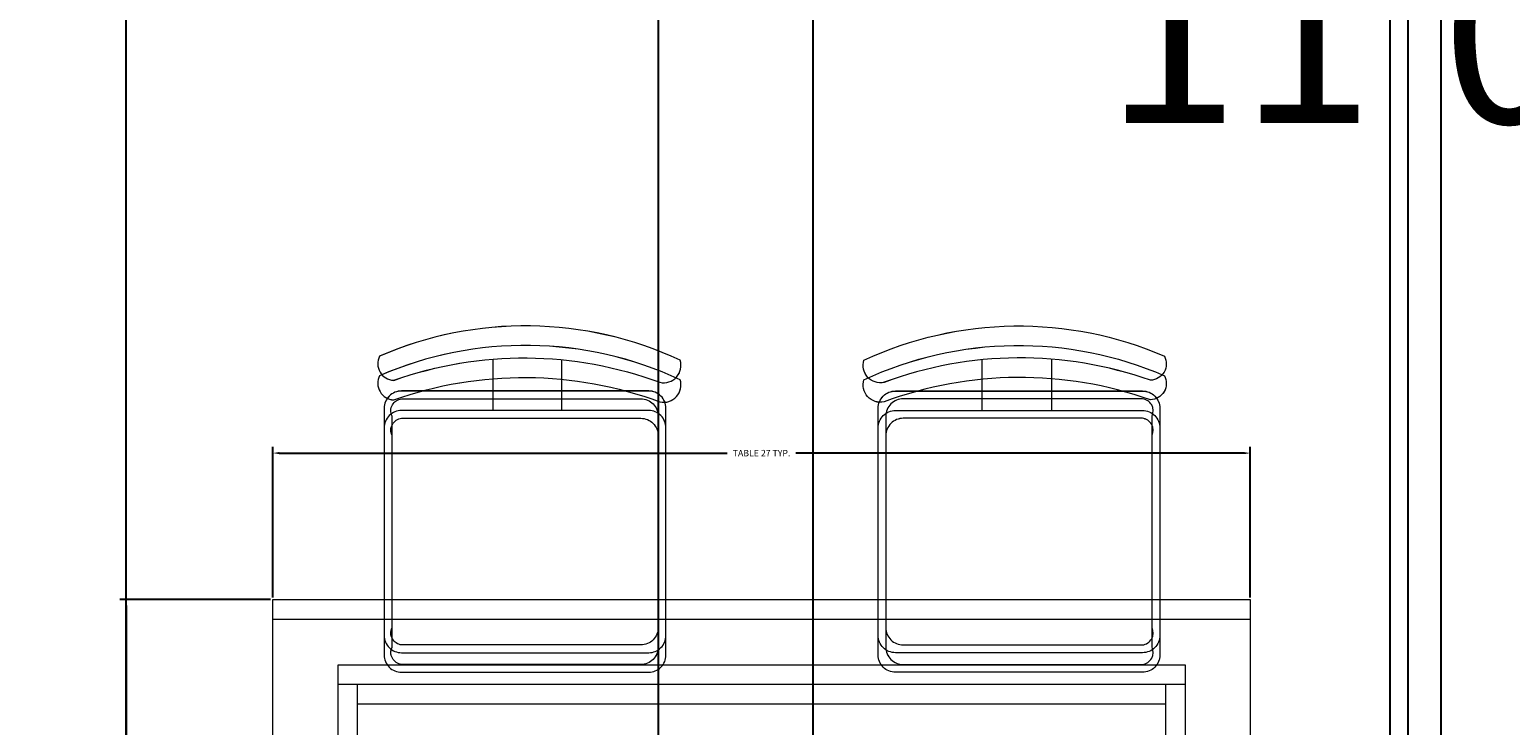
# Model space of a CAD drawing. Units: inches. Extents: x 2063 to 2617, y 1299 to 2210.
# Tile 11 of 22: x 2242 to 2284, y 1925 to 1945. Entities that reach past the tile are written whole.
import ezdxf

# ---------------------------------------------------------------- set-up
doc = ezdxf.new("R2010")
doc.units = ezdxf.units.IN
for name, color, linetype, lineweight in [('A-ANNO-DIMS', 2, 'Continuous', 18), ('A-AREA-IDEN', 7, 'Continuous', 18), ('A-FURN', 8, 'Continuous', 18)]:
    doc.layers.add(name, color=color, linetype=linetype, lineweight=lineweight)
doc.layers.add('A-WALL-PATT', color=215, linetype='Continuous', lineweight=13, true_color=0xa953a0)
doc.styles.get("Standard").update_dxf_attribs({"font": 'arial.ttf'})
doc.dimstyles.get("Standard").update_dxf_attribs({"dimtxt": 0.18, "dimasz": 0.18, "dimexe": 0.18, "dimexo": 0.0625, "dimgap": 0.09, "dimtad": 0, "dimtih": 1, "dimtoh": 1, "dimdec": 4, "dimzin": 0, "dimdsep": 46, "dimtxsty": 'Standard', "dimcen": 0.09, "dimadec": 0, "dimazin": 0, "dimtfac": 1, "dimtdec": 4, "dimtofl": 0, "dimtmove": 0, "dimatfit": 3, "dimfxl": 1, "dimtolj": 1, "dimtzin": 0, "dimarcsym": 0})

# ---------------------------------------------------------------- blocks, each defined once
blk = doc.blocks.new('TABLE-DINING')
for points in [[(0, 17.017), (27.446, 17.017), (27.446, 0.549), (0, 0.549)], [(0, 17.017), (27.446, 17.017), (27.446, 0.549), (0, 0.549)], [(0, 17.016), (27.446, 17.016), (27.446, 0.549), (0, 0.549)], [(0, 17.016), (27.446, 17.016), (27.446, 0.549), (0, 0.549)], [(0, 16.468), (27.446, 16.468), (27.446, 0), (0, 0)], [(0, 16.468), (27.446, 16.468), (27.446, 0), (0, 0)], [(0, 16.467), (27.446, 16.467), (27.446, 0), (0, 0)], [(0, 16.467), (27.446, 16.467), (27.446, 0), (0, 0)], [(1.83, 15.187), (25.616, 15.187), (25.616, 2.379), (1.83, 2.379)], [(1.83, 15.187), (25.616, 15.187), (25.616, 2.379), (1.83, 2.379)], [(1.83, 15.187), (25.616, 15.187), (25.616, 2.379), (1.83, 2.379)], [(1.83, 15.187), (25.616, 15.187), (25.616, 2.379), (1.83, 2.379)], [(1.83, 14.638), (25.616, 14.638), (25.616, 1.83), (1.83, 1.83)], [(1.83, 14.638), (25.616, 14.638), (25.616, 1.83), (1.83, 1.83)], [(1.83, 14.638), (25.616, 14.638), (25.616, 1.83), (1.83, 1.83)], [(1.83, 14.638), (25.616, 14.638), (25.616, 1.83), (1.83, 1.83)], [(2.379, 14.638), (25.067, 14.638), (25.067, 2.928), (2.379, 2.928)], [(2.379, 14.638), (25.067, 14.638), (25.067, 2.927), (2.379, 2.927)], [(2.379, 14.638), (25.067, 14.638), (25.067, 2.928), (2.379, 2.928)], [(2.379, 14.638), (25.067, 14.638), (25.067, 2.927), (2.379, 2.927)], [(2.379, 14.089), (25.067, 14.089), (25.067, 2.379), (2.379, 2.379)], [(2.379, 14.089), (25.067, 14.089), (25.067, 2.379), (2.379, 2.379)], [(2.379, 14.089), (25.067, 14.089), (25.067, 2.379), (2.379, 2.379)], [(2.379, 14.089), (25.067, 14.089), (25.067, 2.379), (2.379, 2.379)]]:
    blk.add_lwpolyline(points, close=True)
blk = doc.blocks.new('CHAIR-DINING')
for points in [[(0.449, 8.202, -0.175809), (7.924, 8.145, 0.578392), (8.491, 8.768, 0.214524), (0.052, 8.881, 0.552014), (0.449, 8.202, -0.065079)], [(0.449, 8.201, -0.175809), (7.924, 8.145, 0.578392), (8.491, 8.767, 0.214524), (0.053, 8.881, 0.552014), (0.449, 8.201, -0.065079)], [(0.449, 8.202, -0.175809), (7.924, 8.145, 0.578392), (8.491, 8.768, 0.214524), (0.052, 8.881, 0.552014), (0.449, 8.202, -0.065079)], [(0.449, 8.201, -0.175809), (7.924, 8.145, 0.578392), (8.491, 8.767, 0.214524), (0.053, 8.881, 0.552014), (0.449, 8.201, -0.065079)], [(0.449, 7.653, -0.175809), (7.924, 7.596, 0.578392), (8.491, 8.219, 0.214524), (0.052, 8.332, 0.552014), (0.449, 7.653, -0.065079)], [(0.449, 7.652, -0.175809), (7.924, 7.596, 0.578392), (8.491, 8.218, 0.214524), (0.053, 8.332, 0.552014), (0.449, 7.652, -0.065079)], [(0.449, 7.653, -0.175809), (7.924, 7.596, 0.578392), (8.491, 8.219, 0.214524), (0.052, 8.332, 0.552014), (0.449, 7.653, -0.065079)], [(0.449, 7.652, -0.175809), (7.924, 7.596, 0.578392), (8.491, 8.218, 0.214524), (0.053, 8.332, 0.552014), (0.449, 7.652, -0.065079)], [(5.17, 7.902), (5.17, 8.779, -0.064759)], [(5.17, 7.901), (5.17, 8.779, -0.064759)], [(5.17, 7.902), (5.17, 8.779, -0.064759)], [(5.17, 7.901), (5.17, 8.779, -0.064759)], [(7.607, 7.902), (0.667, 7.902, 0.414214), (0.182, 7.416), (0.182, 1.035, 0.414214), (0.667, 0.549), (7.607, 0.549, 0.414214), (8.093, 1.035), (8.093, 7.416, 0.414214), (7.607, 7.902)], [(7.607, 7.902), (0.667, 7.902, 0.414214), (0.182, 7.416), (0.182, 1.035, 0.414214), (0.667, 0.549), (7.607, 0.549, 0.414214), (8.093, 1.035), (8.093, 7.416, 0.414214), (7.607, 7.902)], [(7.607, 7.901), (0.667, 7.901, 0.414214), (0.182, 7.416), (0.182, 1.035, 0.414214), (0.667, 0.549), (7.607, 0.549, 0.414214), (8.093, 1.035), (8.093, 7.416, 0.414214), (7.607, 7.901)], [(7.607, 7.901), (0.667, 7.901, 0.414214), (0.182, 7.416), (0.182, 1.035, 0.414214), (0.667, 0.549), (7.607, 0.549, 0.414214), (8.093, 1.035), (8.093, 7.416, 0.414214), (7.607, 7.901)], [(5.17, 7.353), (5.17, 8.23, -0.064759)], [(5.17, 7.352), (5.17, 8.23, -0.064759)], [(5.17, 7.353), (5.17, 8.23, -0.064759)], [(5.17, 7.352), (5.17, 8.23, -0.064759)], [(7.607, 7.353), (0.667, 7.353, 0.414214), (0.182, 6.867), (0.182, 0.486, 0.414214), (0.667, 0), (7.607, 0, 0.414214), (8.093, 0.486), (8.093, 6.867, 0.414214), (7.607, 7.353)], [(7.607, 7.353), (0.667, 7.353, 0.414214), (0.182, 6.867), (0.182, 0.486, 0.414214), (0.667, 0), (7.607, 0, 0.414214), (8.093, 0.486), (8.093, 6.867, 0.414214), (7.607, 7.353)], [(7.607, 7.352), (0.667, 7.352, 0.414214), (0.182, 6.867), (0.182, 0.486, 0.414214), (0.667, 0), (7.607, 0, 0.414214), (8.093, 0.486), (8.093, 6.867, 0.414214), (7.607, 7.352)], [(7.607, 7.352), (0.667, 7.352, 0.414214), (0.182, 6.867), (0.182, 0.486, 0.414214), (0.667, 0), (7.607, 0, 0.414214), (8.093, 0.486), (8.093, 6.867, 0.414214), (7.607, 7.352)]]:
    blk.add_lwpolyline(points, format="xyb")
for points in [[(3.227, 8.795), (3.227, 7.902)], [(3.227, 8.795), (3.227, 7.901)], [(3.227, 8.795), (3.227, 7.902)], [(3.227, 8.795), (3.227, 7.901)], [(3.227, 8.246), (3.227, 7.353)], [(3.227, 8.246), (3.227, 7.352)], [(3.227, 8.246), (3.227, 7.353)], [(3.227, 8.246), (3.227, 7.352)]]:
    blk.add_lwpolyline(points)
for points in [[(0.67, 7.683), (7.388, 7.683, -0.414214), (7.874, 7.197), (7.874, 1.254, -0.414214), (7.388, 0.768), (0.67, 0.768, -0.512069), (0.4, 1.254), (0.4, 7.197, -0.512069)], [(0.67, 7.683), (7.388, 7.683, -0.414214), (7.874, 7.197), (7.874, 1.253, -0.414214), (7.388, 0.768), (0.67, 0.768, -0.512069), (0.4, 1.253), (0.4, 7.197, -0.512069)], [(0.67, 7.683), (7.388, 7.683, -0.414214), (7.874, 7.197), (7.874, 1.254, -0.414214), (7.388, 0.768), (0.67, 0.768, -0.512069), (0.4, 1.254), (0.4, 7.197, -0.512069)], [(0.67, 7.683), (7.388, 7.683, -0.414214), (7.874, 7.197), (7.874, 1.253, -0.414214), (7.388, 0.768), (0.67, 0.768, -0.512069), (0.4, 1.253), (0.4, 7.197, -0.512069)], [(0.67, 7.134), (7.388, 7.134, -0.414214), (7.874, 6.648), (7.874, 0.705, -0.414214), (7.388, 0.219), (0.67, 0.219, -0.512069), (0.4, 0.705), (0.4, 6.648, -0.512069)], [(0.67, 7.134), (7.388, 7.134, -0.414214), (7.874, 6.648), (7.874, 0.704, -0.414214), (7.388, 0.219), (0.67, 0.219, -0.512069), (0.4, 0.704), (0.4, 6.648, -0.512069)], [(0.67, 7.134), (7.388, 7.134, -0.414214), (7.874, 6.648), (7.874, 0.705, -0.414214), (7.388, 0.219), (0.67, 0.219, -0.512069), (0.4, 0.705), (0.4, 6.648, -0.512069)], [(0.67, 7.134), (7.388, 7.134, -0.414214), (7.874, 6.648), (7.874, 0.704, -0.414214), (7.388, 0.219), (0.67, 0.219, -0.512069), (0.4, 0.704), (0.4, 6.648, -0.512069)]]:
    blk.add_lwpolyline(points, format="xyb", close=True)
blk = doc.blocks.new('*D25')
at = {"layer": 'A-ANNO-DIMS', "color": 0, "lineweight": -2, "transparency": 16777216}
for p, q in [((2248.983, 1928.797), (2248.983, 1933.031)), ((2276.429, 1928.797), (2276.429, 1933.031)), ((2249.163, 1932.851), (2261.742, 1932.851)), ((2276.249, 1932.851), (2263.67, 1932.851))]:
    blk.add_line(p, q, dxfattribs=at)
at = {"layer": 'A-ANNO-DIMS', "color": 0, "transparency": 16777216}
for points in [[(2249.163, 1932.881), (2249.163, 1932.821), (2248.983, 1932.851)], [(2276.249, 1932.881), (2276.249, 1932.821), (2276.429, 1932.851)]]:
    blk.add_solid(points, dxfattribs=at)
at = {"layer": 'Defpoints', "color": 0, "transparency": 16777216}
for p in [(2276.429, 1932.851), (2248.983, 1928.735), (2276.429, 1928.735)]:
    blk.add_point(p, dxfattribs=at)
at = {"layer": 'A-ANNO-DIMS', "color": 0, "transparency": 16777216, "insert": (2262.706, 1932.851), "char_height": 0.18, "attachment_point": 5}
blk.add_mtext('\\A1;TABLE 27 TYP.', dxfattribs=at)
blk = doc.blocks.new('*D26')
at = {"layer": 'A-ANNO-DIMS', "color": 0, "lineweight": -2, "transparency": 16777216}
for p, q in [((2248.921, 1928.735), (2244.686, 1928.735)), ((2244.866, 1928.555), (2244.866, 1920.407)), ((2244.866, 1911.898), (2244.866, 1920.046)), ((2248.921, 1911.718), (2244.686, 1911.718))]:
    blk.add_line(p, q, dxfattribs=at)
at = {"layer": 'A-ANNO-DIMS', "color": 0, "transparency": 16777216}
for points in [[(2244.836, 1928.555), (2244.896, 1928.555), (2244.866, 1928.735)], [(2244.836, 1911.898), (2244.896, 1911.898), (2244.866, 1911.718)]]:
    blk.add_solid(points, dxfattribs=at)
at = {"layer": 'Defpoints', "color": 0, "transparency": 16777216}
for p in [(2244.866, 1928.735), (2248.983, 1928.735), (2248.983, 1911.718)]:
    blk.add_point(p, dxfattribs=at)
at = {"layer": 'A-ANNO-DIMS', "color": 0, "transparency": 16777216, "insert": (2244.866, 1920.226), "char_height": 0.18, "attachment_point": 5}
blk.add_mtext('\\A1;17 TYP.', dxfattribs=at)
blk = doc.blocks.new('*D50')
at = {"layer": 'A-ANNO-DIMS', "color": 0, "lineweight": -2, "transparency": 16777216}
for p, q in [((2264.144, 2124.25), (2264.144, 1317.702)), ((2280.348, 2124.25), (2280.348, 1317.702)), ((2264.324, 1317.882), (2271.791, 1317.882)), ((2280.168, 1317.882), (2272.701, 1317.882))]:
    blk.add_line(p, q, dxfattribs=at)
at = {"layer": 'A-ANNO-DIMS', "color": 0, "transparency": 16777216}
for points in [[(2264.324, 1317.912), (2264.324, 1317.852), (2264.144, 1317.882)], [(2280.168, 1317.912), (2280.168, 1317.852), (2280.348, 1317.882)]]:
    blk.add_solid(points, dxfattribs=at)
at = {"layer": 'Defpoints', "color": 0, "transparency": 16777216}
for p in [(2264.144, 2124.312), (2280.348, 2124.312), (2280.348, 1317.882)]:
    blk.add_point(p, dxfattribs=at)
at = {"layer": 'A-ANNO-DIMS', "color": 0, "transparency": 16777216, "insert": (2272.246, 1317.882), "char_height": 0.18, "attachment_point": 5}
blk.add_mtext('\\A1;16.204', dxfattribs=at)
blk = doc.blocks.new('*D62')
at = {"layer": 'A-ANNO-DIMS', "color": 0, "lineweight": -2, "transparency": 16777216}
for p, q in [((2259.809, 1437.875), (2259.809, 2170.742)), ((2259.989, 2170.562), (2270.403, 2170.562)), ((2281.608, 2170.562), (2271.194, 2170.562)), ((2281.788, 1437.875), (2281.788, 2170.742))]:
    blk.add_line(p, q, dxfattribs=at)
at = {"layer": 'A-ANNO-DIMS', "color": 0, "transparency": 16777216}
for points in [[(2259.989, 2170.592), (2259.989, 2170.532), (2259.809, 2170.562)], [(2281.608, 2170.592), (2281.608, 2170.532), (2281.788, 2170.562)]]:
    blk.add_solid(points, dxfattribs=at)
at = {"layer": 'Defpoints', "color": 0, "transparency": 16777216}
for p in [(2281.788, 2170.562), (2259.809, 1437.812), (2281.788, 1437.812)]:
    blk.add_point(p, dxfattribs=at)
at = {"layer": 'A-ANNO-DIMS', "color": 0, "transparency": 16777216, "insert": (2270.798, 2170.562), "char_height": 0.18, "attachment_point": 5}
blk.add_mtext('\\A1;21.98', dxfattribs=at)
blk = doc.blocks.new('*D63')
at = {"layer": 'A-ANNO-DIMS', "color": 0, "lineweight": -2, "transparency": 16777216}
for p, q in [((2244.867, 1562.375), (2244.867, 2170.742)), ((2245.047, 2170.562), (2262.4, 2170.562)), ((2280.682, 2170.562), (2263.329, 2170.562)), ((2280.862, 1562.375), (2280.862, 2170.742))]:
    blk.add_line(p, q, dxfattribs=at)
at = {"layer": 'A-ANNO-DIMS', "color": 0, "transparency": 16777216}
for points in [[(2245.047, 2170.592), (2245.047, 2170.532), (2244.867, 2170.562)], [(2280.682, 2170.592), (2280.682, 2170.532), (2280.862, 2170.562)]]:
    blk.add_solid(points, dxfattribs=at)
at = {"layer": 'Defpoints', "color": 0, "transparency": 16777216}
for p in [(2280.862, 2170.562), (2244.867, 1562.312), (2280.862, 1562.312)]:
    blk.add_point(p, dxfattribs=at)
at = {"layer": 'A-ANNO-DIMS', "color": 0, "transparency": 16777216, "insert": (2262.865, 2170.562), "char_height": 0.18, "attachment_point": 5}
blk.add_mtext('\\A1;35.995', dxfattribs=at)

msp = doc.modelspace()

# ---------------------------------------------------------------- hatches: boundary and pattern name
at = {"layer": 'A-WALL-PATT'}
h = msp.add_hatch(dxfattribs=at)
h.set_pattern_fill('ANSI32', color=256)
h.paths.add_polyline_path([(2553.6442, 2128.8122), (2511.1703, 2128.8122), (2511.1703, 2124.3122), (2549.1442, 2124.3122), (2549.1442, 2095.662), (2553.6442, 2095.662)])
h.paths.add_polyline_path([(2553.6442, 2035.662), (2549.1442, 2035.662), (2549.1442, 1980.3122), (2503.7214, 1980.3122), (2503.7214, 1975.8122), (2549.1442, 1975.8122), (2549.1442, 1962.9693), (2553.6442, 1962.9693)])
h.paths.add_polyline_path([(2553.6442, 1938.9693), (2549.1442, 1938.9693), (2549.1442, 1927.8122), (2477.1442, 1927.8122), (2477.1442, 1975.8122), (2481.2918, 1975.8122), (2481.2918, 1980.3122), (2453.2648, 1980.3122), (2453.2648, 1975.8122), (2472.6442, 1975.8122), (2472.6442, 1868.3122), (2400.6442, 1868.3122), (2400.6442, 1861.3782), (2405.1442, 1861.3782), (2405.1442, 1863.8122), (2480.9699, 1863.8122), (2480.9699, 1866.0622), (2480.9699, 1868.3122), (2477.1442, 1868.3122), (2477.1442, 1923.3122), (2549.1442, 1923.3122), (2549.1442, 1908.8504), (2553.6442, 1908.8504)])
h.paths.add_polyline_path([(2553.6442, 1884.8504), (2549.1442, 1884.8504), (2549.1442, 1868.3122), (2501.0636, 1868.3122), (2501.0636, 1863.8122), (2549.1442, 1863.8122), (2549.1442, 1826.0298), (2553.6442, 1826.0298)])
h.paths.add_polyline_path([(2388.1504, 1980.3122), (2340.6442, 1980.3122), (2340.6442, 2124.3122), (2358.7501, 2124.3122), (2358.7501, 2128.8122), (2316.3482, 2128.8122), (2316.3482, 2124.3122), (2336.1442, 2124.3122), (2336.1442, 1980.3122), (2289.1737, 1980.3122), (2289.1737, 1975.8122), (2336.1442, 1975.8122), (2336.1442, 1619.3122), (2333.1433, 1619.3122), (2333.1433, 1614.8122), (2344.1671, 1614.8122), (2344.1671, 1617.0622), (2344.1671, 1619.3122), (2340.6442, 1619.3122), (2340.6442, 1975.8122), (2388.1504, 1975.8122), (2388.1504, 1978.0622)])
h.paths.add_polyline_path([(2290.1442, 1614.8122), (2301.4594, 1614.8122), (2301.4594, 1617.0622), (2301.4594, 1619.3122), (2285.6442, 1619.3122), (2285.6442, 1566.8122), (2280.8619, 1566.8122), (2280.8619, 1564.5622), (2280.8619, 1562.3122), (2285.6442, 1562.3122), (2285.6442, 1442.3122), (2281.7879, 1442.3122), (2281.7879, 1437.8122), (2285.6442, 1437.8122), (2285.6442, 1401.8122), (2290.1442, 1401.8122)])
h.paths.add_polyline_path([(2549.1442, 1731.8122), (2405.1442, 1731.8122), (2405.1442, 1834.4638), (2402.8942, 1834.4638), (2400.6442, 1834.4638), (2400.6442, 1727.3122), (2549.1442, 1727.3122)])
h.paths.add_polyline_path([(2553.6442, 1766.0298), (2551.3942, 1766.0298), (2549.1442, 1766.0298), (2549.1442, 1686.7767), (2553.6442, 1686.7767)])
h.paths.add_polyline_path([(2553.6442, 1638.7767), (2551.3942, 1638.7767), (2549.1442, 1638.7767), (2549.1442, 1619.3122), (2448.6442, 1619.3122), (2448.6442, 1610.5671), (2450.8942, 1610.5671), (2453.1442, 1610.5671), (2453.1442, 1614.8122), (2549.1442, 1614.8122), (2549.1442, 1601.6421), (2553.6442, 1601.6421)])
h.paths.add_polyline_path([(2553.6442, 1577.6421), (2551.3942, 1577.6421), (2549.1442, 1577.6421), (2549.1442, 1566.8122), (2453.1442, 1566.8122), (2453.1442, 1591.5045), (2451.0335, 1591.5045), (2448.6442, 1591.5045), (2448.6442, 1566.8122), (2434.0475, 1566.8122), (2434.0475, 1562.3122), (2549.1442, 1562.3122), (2549.1442, 1533.48), (2553.6442, 1533.48)])
h.paths.add_polyline_path([(2553.6442, 1473.48), (2549.1442, 1473.48), (2549.1442, 1442.3122), (2502.6258, 1442.3122), (2502.6258, 1437.8122), (2549.1442, 1437.8122), (2549.1442, 1401.8122), (2553.6442, 1401.8122)])
h.paths.add_polyline_path([(2395.6442, 1562.3122), (2400.0901, 1562.3122), (2400.0901, 1564.5622), (2400.0901, 1566.8122), (2395.6442, 1566.8122), (2395.6442, 1619.3122), (2379.1127, 1619.3122), (2379.1127, 1614.8122), (2391.1442, 1614.8122), (2391.1442, 1401.8122), (2395.6442, 1401.8122), (2395.6442, 1437.8122), (2399.2425, 1437.8122), (2399.2425, 1440.0622), (2399.2425, 1442.3122), (2395.6442, 1442.3122)])
h.paths.add_polyline_path([(2442.6258, 1442.3122), (2419.6262, 1442.3122), (2419.6262, 1437.8122), (2442.6258, 1437.8122), (2442.6258, 1440.0622)])
h.paths.add_polyline_path([(2127.6442, 1480.2532), (2125.3942, 1480.2532), (2123.1442, 1480.2532), (2123.1442, 1401.8122), (2127.6442, 1401.8122), (2127.6442, 1437.8122), (2145.1538, 1437.8122), (2145.1538, 1440.0622), (2145.1538, 1442.3122), (2127.6442, 1442.3122)])
h.paths.add_polyline_path([(2259.809, 1442.3122), (2205.1538, 1442.3122), (2205.1538, 1437.8122), (2259.809, 1437.8122), (2259.809, 1440.0622)])
h.paths.add_polyline_path([(2127.6442, 1659.7652), (2123.1442, 1659.7652), (2123.1442, 1605.5161), (2125.3942, 1605.5161), (2127.6442, 1605.5161), (2127.6442, 1614.8122), (2223.6442, 1614.8122), (2223.6442, 1611.2723), (2228.1442, 1611.2723), (2228.1442, 1619.3122), (2127.6442, 1619.3122)])
h.paths.add_polyline_path([(2244.8673, 1566.8122), (2228.1442, 1566.8122), (2228.1442, 1590.8122), (2225.8942, 1590.8122), (2223.6442, 1590.8122), (2223.6442, 1566.8122), (2127.6442, 1566.8122), (2127.6442, 1581.5161), (2123.1442, 1581.5161), (2123.1442, 1540.2532), (2127.6442, 1540.2532), (2127.6442, 1562.3122), (2244.8673, 1562.3122), (2244.8673, 1564.5622)])
h.paths.add_polyline_path([(2172.5174, 1868.3122), (2127.6442, 1868.3122), (2127.6442, 1886.5833), (2123.1442, 1886.5833), (2123.1442, 1832.6633), (2127.6442, 1832.6633), (2127.6442, 1863.8122), (2172.5174, 1863.8122), (2172.5174, 1866.0622)])
h.paths.add_polyline_path([(2276.1442, 1868.3122), (2204.1442, 1868.3122), (2204.1442, 1923.3122), (2204.1442, 1975.8122), (2224.8362, 1975.8122), (2224.8362, 1978.1097), (2224.8362, 1980.3122), (2195.0729, 1980.3122), (2195.0729, 1978.0622), (2195.0729, 1975.8122), (2199.6442, 1975.8122), (2199.6442, 1927.8122), (2127.6442, 1927.8122), (2127.6442, 1942.3492), (2123.1442, 1942.3492), (2123.1442, 1910.5833), (2127.6442, 1910.5833), (2127.6442, 1923.3122), (2199.6442, 1923.3122), (2199.6442, 1868.3122), (2194.8228, 1868.3122), (2194.8228, 1864.7337), (2194.8228, 1863.8122), (2271.6442, 1863.8122), (2271.6442, 1860.0507), (2276.1442, 1860.0507)])
h.paths.add_polyline_path([(2276.1442, 1829.994), (2273.8942, 1829.994), (2271.6442, 1829.994), (2271.6442, 1731.8122), (2127.6442, 1731.8122), (2127.6442, 1772.6633), (2123.1442, 1772.6633), (2123.1442, 1707.7652), (2127.6442, 1707.7652), (2127.6442, 1727.3122), (2276.1442, 1727.3122)])
h.paths.add_polyline_path([(2127.6442, 2022.1152), (2123.1442, 2022.1152), (2123.1442, 1966.3492), (2127.6442, 1966.3492), (2127.6442, 1975.8122), (2174.2082, 1975.8122), (2174.2082, 1978.0622), (2174.2082, 1980.3122), (2127.6442, 1980.3122)])
h.paths.add_polyline_path([(2361.9755, 1678.588), (2398.4558, 1678.588), (2398.4558, 1697.2453), (2361.9755, 1697.2453)], flags=9)
h.paths.add_polyline_path([(2351.5397, 1780.4072), (2386.1987, 1780.4072), (2386.1987, 1790.7107), (2351.5397, 1790.7107)], flags=25)
h.paths.add_polyline_path([(2350.6753, 1940.9321), (2387.6024, 1940.9321), (2387.6024, 1959.5894), (2350.6753, 1959.5894)], flags=25)
h.paths.add_polyline_path([(2254.9545, 1684.638), (2295.0943, 1684.638), (2295.0943, 1703.2953), (2254.9545, 1703.2953)], flags=9)
h.paths.add_polyline_path([(2282.4946, 1782.4438), (2317.1535, 1782.4438), (2317.1535, 1792.7474), (2282.4946, 1792.7474)], flags=9)
h.paths.add_polyline_path([(2270.327, 1939.2854), (2307.254, 1939.2854), (2307.254, 1957.9428), (2270.327, 1957.9428)], flags=9)

# ---------------------------------------------------------------- linework, layer by layer
at = {"layer": 'A-FURN'}
for points in [[(2266.1467, 1934.839, -0.5783921), (2265.5804, 1935.4617, -0.2145244), (2274.0186, 1935.5749, -0.552014), (2273.6222, 1934.8956, 0.1758092), (2266.1467, 1934.839)], [(2266.1467, 1934.839, -0.5783921), (2265.5804, 1935.4617, -0.2145244), (2274.0186, 1935.5749, -0.552014), (2273.6222, 1934.8956, 0.1758092), (2266.1467, 1934.839)], [(2266.1467, 1934.8387, -0.5783921), (2265.5804, 1935.4614, -0.2145244), (2274.0186, 1935.5746, -0.552014), (2273.6222, 1934.8953, 0.1758092), (2266.1467, 1934.8387)], [(2266.1467, 1934.8387, -0.5783921), (2265.5804, 1935.4614, -0.2145244), (2274.0186, 1935.5746, -0.552014), (2273.6222, 1934.8953, 0.1758092), (2266.1467, 1934.8387)], [(2266.1467, 1934.2901, -0.5783921), (2265.5804, 1934.9128, -0.2145244), (2274.0186, 1935.026, -0.552014), (2273.6222, 1934.3467, 0.1758092), (2266.1467, 1934.2901)], [(2266.1467, 1934.2901, -0.5783921), (2265.5804, 1934.9128, -0.2145244), (2274.0186, 1935.026, -0.552014), (2273.6222, 1934.3467, 0.1758092), (2266.1467, 1934.2901)], [(2266.1467, 1934.2898, -0.5783921), (2265.5804, 1934.9125, -0.2145244), (2274.0186, 1935.0257, -0.552014), (2273.6222, 1934.3464, 0.1758092), (2266.1467, 1934.2898)], [(2266.1467, 1934.2898, -0.5783921), (2265.5804, 1934.9125, -0.2145244), (2274.0186, 1935.0257, -0.552014), (2273.6222, 1934.3464, 0.1758092), (2266.1467, 1934.2898)], [(2268.9015, 1934.5956), (2268.9015, 1935.4732, 0.0647586)], [(2268.9015, 1934.5956), (2268.9015, 1935.4732, 0.0647586)], [(2268.9015, 1934.5953), (2268.9015, 1935.473, 0.0647586)], [(2268.9015, 1934.5953), (2268.9015, 1935.473, 0.0647586)], [(2268.9015, 1934.0466), (2268.9015, 1934.9243, 0.0647586)], [(2268.9015, 1934.0466), (2268.9015, 1934.9243, 0.0647586)], [(2268.9015, 1934.0464), (2268.9015, 1934.924, 0.0647586)], [(2268.9015, 1934.0464), (2268.9015, 1934.924, 0.0647586)], [(2273.4038, 1934.5956, -0.4142136), (2273.8893, 1934.11), (2273.8893, 1927.7289, -0.4142136), (2273.4038, 1927.2434), (2266.4639, 1927.2434, -0.4142136), (2265.9783, 1927.7289), (2265.9783, 1934.11, -0.4142136), (2266.4639, 1934.5956), (2273.4038, 1934.5956)], [(2273.4038, 1934.5956, -0.4142136), (2273.8893, 1934.11), (2273.8893, 1927.7289, -0.4142136), (2273.4038, 1927.2434), (2266.4639, 1927.2434, -0.4142136), (2265.9783, 1927.7289), (2265.9783, 1934.11, -0.4142136), (2266.4639, 1934.5956), (2273.4038, 1934.5956)], [(2273.4038, 1934.5953, -0.4142136), (2273.8893, 1934.1097), (2273.8893, 1927.7286, -0.4142136), (2273.4038, 1927.2431), (2266.4639, 1927.2431, -0.4142136), (2265.9784, 1927.7286), (2265.9784, 1934.1097, -0.4142136), (2266.4639, 1934.5953), (2273.4038, 1934.5953)], [(2273.4038, 1934.5953, -0.4142136), (2273.8893, 1934.1097), (2273.8893, 1927.7286, -0.4142136), (2273.4038, 1927.2431), (2266.4639, 1927.2431, -0.4142136), (2265.9784, 1927.7286), (2265.9784, 1934.1097, -0.4142136), (2266.4639, 1934.5953), (2273.4038, 1934.5953)], [(2273.4038, 1934.0466, -0.4142136), (2273.8893, 1933.5611), (2273.8893, 1927.18, -0.4142136), (2273.4038, 1926.6944), (2266.4639, 1926.6944, -0.4142136), (2265.9783, 1927.18), (2265.9783, 1933.5611, -0.4142136), (2266.4639, 1934.0466), (2273.4038, 1934.0466)], [(2273.4038, 1934.0466, -0.4142136), (2273.8893, 1933.5611), (2273.8893, 1927.18, -0.4142136), (2273.4038, 1926.6944), (2266.4639, 1926.6944, -0.4142136), (2265.9783, 1927.18), (2265.9783, 1933.5611, -0.4142136), (2266.4639, 1934.0466), (2273.4038, 1934.0466)], [(2273.4038, 1934.0464, -0.4142136), (2273.8893, 1933.5608), (2273.8893, 1927.1797, -0.4142136), (2273.4038, 1926.6942), (2266.4639, 1926.6942, -0.4142136), (2265.9784, 1927.1797), (2265.9784, 1933.5608, -0.4142136), (2266.4639, 1934.0464), (2273.4038, 1934.0464)], [(2273.4038, 1934.0464, -0.4142136), (2273.8893, 1933.5608), (2273.8893, 1927.1797, -0.4142136), (2273.4038, 1926.6942), (2266.4639, 1926.6942, -0.4142136), (2265.9784, 1927.1797), (2265.9784, 1933.5608, -0.4142136), (2266.4639, 1934.0464), (2273.4038, 1934.0464)]]:
    msp.add_lwpolyline(points, format="xyb", dxfattribs=at)
for points in [[(2270.8441, 1935.4892), (2270.8441, 1934.5956)], [(2270.8441, 1935.4892), (2270.8441, 1934.5956)], [(2270.8441, 1935.4889), (2270.8441, 1934.5953)], [(2270.8441, 1935.4889), (2270.8441, 1934.5953)], [(2270.8441, 1934.9403), (2270.8441, 1934.0466)], [(2270.8441, 1934.9403), (2270.8441, 1934.0466)], [(2270.8441, 1934.94), (2270.8441, 1934.0464)], [(2270.8441, 1934.94), (2270.8441, 1934.0464)]]:
    msp.add_lwpolyline(points, dxfattribs=at)
for points in [[(2273.4009, 1934.3768), (2266.6826, 1934.3768, 0.4142136), (2266.1971, 1933.8913), (2266.1971, 1927.9476, 0.4142136), (2266.6826, 1927.4621), (2273.4009, 1927.4621, 0.5120695), (2273.6706, 1927.9476), (2273.6706, 1933.8913, 0.5120695)], [(2273.4009, 1934.3768), (2266.6826, 1934.3768, 0.4142136), (2266.1971, 1933.8913), (2266.1971, 1927.9476, 0.4142136), (2266.6826, 1927.4621), (2273.4009, 1927.4621, 0.5120695), (2273.6706, 1927.9476), (2273.6706, 1933.8913, 0.5120695)], [(2273.4009, 1934.3765), (2266.6826, 1934.3765, 0.4142136), (2266.1971, 1933.891), (2266.1971, 1927.9473, 0.4142136), (2266.6826, 1927.4618), (2273.4009, 1927.4618, 0.5120695), (2273.6706, 1927.9473), (2273.6706, 1933.891, 0.5120695)], [(2273.4009, 1934.3765), (2266.6826, 1934.3765, 0.4142136), (2266.1971, 1933.891), (2266.1971, 1927.9473, 0.4142136), (2266.6826, 1927.4618), (2273.4009, 1927.4618, 0.5120695), (2273.6706, 1927.9473), (2273.6706, 1933.891, 0.5120695)], [(2273.4009, 1933.8279), (2266.6826, 1933.8279, 0.4142136), (2266.1971, 1933.3424), (2266.1971, 1927.3987, 0.4142136), (2266.6826, 1926.9132), (2273.4009, 1926.9132, 0.5120695), (2273.6706, 1927.3987), (2273.6706, 1933.3424, 0.5120695)], [(2273.4009, 1933.8279), (2266.6826, 1933.8279, 0.4142136), (2266.1971, 1933.3424), (2266.1971, 1927.3987, 0.4142136), (2266.6826, 1926.9132), (2273.4009, 1926.9132, 0.5120695), (2273.6706, 1927.3987), (2273.6706, 1933.3424, 0.5120695)], [(2273.4009, 1933.8276), (2266.6826, 1933.8276, 0.4142136), (2266.1971, 1933.3421), (2266.1971, 1927.3984, 0.4142136), (2266.6826, 1926.9129), (2273.4009, 1926.9129, 0.5120695), (2273.6706, 1927.3984), (2273.6706, 1933.3421, 0.5120695)], [(2273.4009, 1933.8276), (2266.6826, 1933.8276, 0.4142136), (2266.1971, 1933.3421), (2266.1971, 1927.3984, 0.4142136), (2266.6826, 1926.9129), (2273.4009, 1926.9129, 0.5120695), (2273.6706, 1927.3984), (2273.6706, 1933.3421, 0.5120695)]]:
    msp.add_lwpolyline(points, format="xyb", close=True, dxfattribs=at)

# ---------------------------------------------------------------- block references
for name, p in [('CHAIR-DINING', (2251.929, 1926.694)), ('TABLE-DINING', (2248.983, 1911.718))]:
    msp.add_blockref(name, p, dxfattribs=at)

# ---------------------------------------------------------------- texts
at = {"layer": 'A-AREA-IDEN', "insert": (2272.3376, 1955.4547), "char_height": 5, "attachment_point": 1}
msp.add_mtext_dynamic_manual_height_columns('DINING\\P11\'0"x10\'0"  ', width=126.60671, gutter_width=12.5, heights=[0], dxfattribs=at)

# ---------------------------------------------------------------- dimensions: what is measured, and where the dimension line sits
at = {"layer": 'A-ANNO-DIMS'}
for base, p1, p2, override, picture, middle in [((2280.8619, 2170.5622), (2244.8673, 1562.3122), (2280.8619, 1562.3122), {"dimdec": 3, "dimlfac": 1, "dimrnd": 0, "dimzin": 0, "dimdsep": 46, "dimlunit": 2}, '*D63', (2262.8646, 2170.5622)), ((2281.7879, 2170.5622), (2259.809, 1437.8122), (2281.7879, 1437.8122), {"dimdec": 2, "dimlfac": 1, "dimrnd": 0, "dimzin": 0, "dimdsep": 46, "dimlunit": 2}, '*D62', (2270.7984, 2170.5622)), ((2280.3482, 1317.8821), (2264.1442, 2124.3122), (2280.3482, 2124.3122), {"dimdec": 3, "dimlfac": 1, "dimrnd": 0, "dimzin": 0, "dimdsep": 46, "dimlunit": 2}, '*D50', (2272.2462, 1317.8821))]:
    dim = msp.add_linear_dim(base=base, p1=p1, p2=p2, dimstyle='Standard', override=override, dxfattribs=at)
    dim.commit()
    dim.dimension.update_dxf_attribs({"geometry": picture, "text_midpoint": middle})
dim = msp.add_linear_dim(base=(2276.4289, 1932.8515), p1=(2248.9832, 1928.7346), p2=(2276.4289, 1928.7346), text='TABLE <> TYP.', dimstyle='Standard', override={"dimdec": 0, "dimlfac": 1, "dimrnd": 0, "dimzin": 0, "dimdsep": 46, "dimlunit": 2}, dxfattribs=at)
dim.commit()
dim.dimension.update_dxf_attribs({"geometry": '*D25', "text_midpoint": (2262.706, 1932.8515)})
dim = msp.add_linear_dim(base=(2244.8663, 1928.7346), p1=(2248.9832, 1911.718), p2=(2248.9832, 1928.7346), angle=90, text='<> TYP.', dimstyle='Standard', override={"dimdec": 0, "dimlfac": 1, "dimrnd": 0, "dimzin": 0, "dimdsep": 46, "dimlunit": 2}, dxfattribs=at)
dim.commit()
dim.dimension.update_dxf_attribs({"geometry": '*D26', "text_midpoint": (2244.8663, 1920.2263)})

doc.saveas('drawing.dxf')
